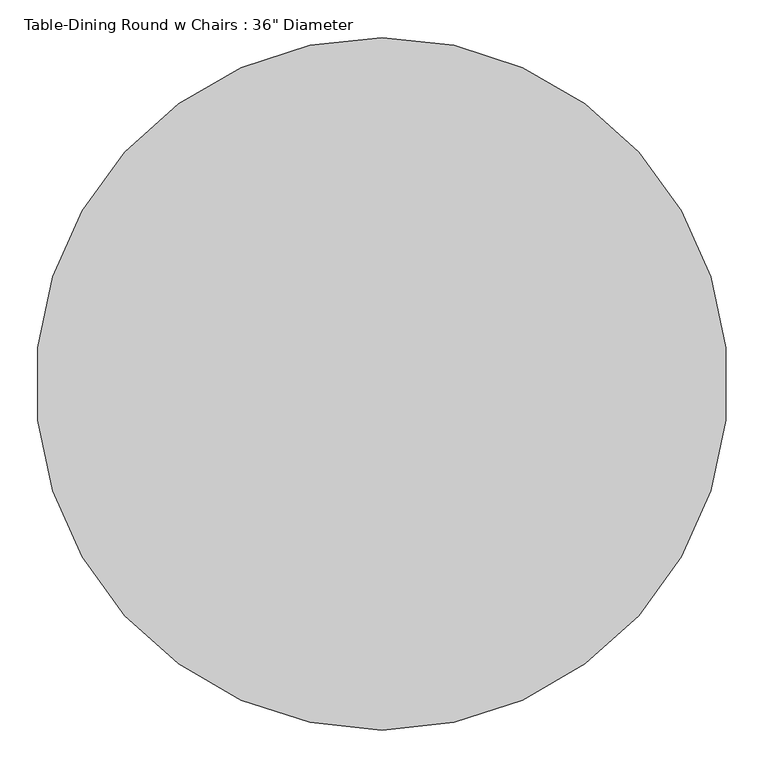
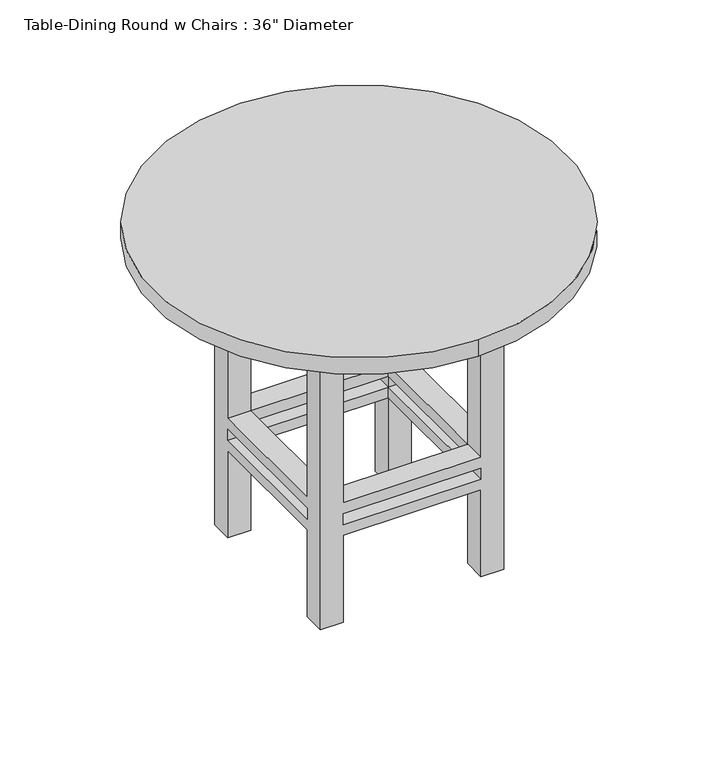
"""IFC4 building model written with IfcOpenShell, lengths in millimetres: furniture geometry."""

from ifc_helpers import new_model, si_unit, point, frame, frame_2d, origin, place, context, project, spatial, polyline, circle_curve, trimmed, segment, composite_curve, outline, extrude, faceted_brep, source, transform, mapped, element, save


def furniture_52f35bf4(model_context):
    return source(origin(), model_context, "Body", "SolidModel", [
        extrude(outline(polyline([(332.2819672, 43.7213115), (332.2819672, -413.4786885), (-124.9180328, -413.4786885), (-124.9180328, 43.7213115), (332.2819672, 43.7213115)]), holes=[polyline([(306.8819672, 18.3213115), (-99.5180328, 18.3213115), (-99.5180328, -388.0786885), (306.8819672, -388.0786885), (306.8819672, 18.3213115)])]), frame((0.0, 0.0, 647.7), z_axis=(0.0, 0.0, 1.0), x_axis=(1.0, 0.0, 0.0)), (0.0, 0.0, 1.0), 76.2),
        faceted_brep([(256.0819672, -32.4786885, 279.4), (256.0819672, -337.2786885, 279.4), (306.8819672, -337.2786885, 279.4), (306.8819672, -32.4786885, 279.4), (-48.7180328, -337.2786885, 279.4), (-48.7180328, -388.0786885, 279.4), (256.0819672, -388.0786885, 279.4), (-48.7180328, -32.4786885, 279.4), (-99.5180328, -32.4786885, 279.4), (-99.5180328, -337.2786885, 279.4), (256.0819672, 18.3213115, 279.4), (-48.7180328, 18.3213115, 279.4), (256.0819672, -32.4786885, 254.0), (-48.7180328, -32.4786885, 254.0), (-48.7180328, 18.3213115, 254.0), (256.0819672, 18.3213115, 254.0), (-48.7180328, -337.2786885, 254.0), (-99.5180328, -337.2786885, 254.0), (-99.5180328, -32.4786885, 254.0), (256.0819672, -337.2786885, 254.0), (256.0819672, -388.0786885, 254.0), (-48.7180328, -388.0786885, 254.0), (306.8819672, -32.4786885, 254.0), (306.8819672, -337.2786885, 254.0), (-99.5180328, 18.3213115, 647.7), (-48.7180328, 18.3213115, 647.7), (256.0819672, 18.3213115, 647.7), (306.8819672, 18.3213115, 647.7), (306.8819672, 18.3213115, 0.0), (256.0819672, 18.3213115, 0.0), (256.0819672, 18.3213115, 203.2), (-48.7180328, 18.3213115, 203.2), (-48.7180328, 18.3213115, 0.0), (-99.5180328, 18.3213115, 0.0), (-48.7180328, 18.3213115, 228.6), (256.0819672, 18.3213115, 228.6), (-99.5180328, -32.4786885, 647.7), (-99.5180328, -32.4786885, 0.0), (-99.5180328, -32.4786885, 203.2), (-99.5180328, -337.2786885, 203.2), (-99.5180328, -337.2786885, 0.0), (-99.5180328, -388.0786885, 0.0), (-99.5180328, -388.0786885, 647.7), (-99.5180328, -337.2786885, 647.7), (-99.5180328, -337.2786885, 228.6), (-99.5180328, -32.4786885, 228.6), (306.8819672, -388.0786885, 647.7), (256.0819672, -388.0786885, 647.7), (-48.7180328, -388.0786885, 647.7), (-48.7180328, -388.0786885, 0.0), (-48.7180328, -388.0786885, 203.2), (256.0819672, -388.0786885, 203.2), (256.0819672, -388.0786885, 0.0), (306.8819672, -388.0786885, 0.0), (256.0819672, -388.0786885, 228.6), (-48.7180328, -388.0786885, 228.6), (306.8819672, -32.4786885, 647.7), (306.8819672, -337.2786885, 647.7), (306.8819672, -337.2786885, 0.0), (306.8819672, -337.2786885, 203.2), (306.8819672, -32.4786885, 203.2), (306.8819672, -32.4786885, 0.0), (306.8819672, -32.4786885, 228.6), (306.8819672, -337.2786885, 228.6), (-48.7180328, -32.4786885, 647.7), (256.0819672, -337.2786885, 647.7), (256.0819672, -32.4786885, 647.7), (-48.7180328, -337.2786885, 647.7), (256.0819672, -32.4786885, 0.0), (-48.7180328, -337.2786885, 0.0), (-48.7180328, -32.4786885, 0.0), (256.0819672, -337.2786885, 0.0), (-48.7180328, -32.4786885, 228.6), (-48.7180328, -32.4786885, 203.2), (256.0819672, -32.4786885, 228.6), (256.0819672, -32.4786885, 203.2), (256.0819672, -337.2786885, 228.6), (256.0819672, -337.2786885, 203.2), (-48.7180328, -337.2786885, 228.6), (-48.7180328, -337.2786885, 203.2)], [[[0, 1, 2, 3]], [[1, 4, 5, 6]], [[4, 7, 8, 9]], [[7, 0, 10, 11]], [[12, 13, 14, 15]], [[13, 16, 17, 18]], [[16, 19, 20, 21]], [[19, 12, 22, 23]], [[24, 25, 11, 10, 26, 27, 28, 29, 30, 31, 32, 33], [14, 34, 35, 15]], [[36, 24, 33, 37, 38, 39, 40, 41, 42, 43, 9, 8], [17, 44, 45, 18]], [[46, 47, 6, 5, 48, 42, 41, 49, 50, 51, 52, 53], [20, 54, 55, 21]], [[28, 27, 56, 3, 2, 57, 46, 53, 58, 59, 60, 61], [22, 62, 63, 23]], [[1, 0, 12, 19]], [[4, 1, 19, 16]], [[7, 4, 16, 13]], [[0, 7, 13, 12]], [[25, 24, 36, 64]], [[47, 46, 57, 65]], [[26, 66, 56, 27]], [[48, 67, 43, 42]], [[29, 28, 61, 68]], [[49, 41, 40, 69]], [[32, 70, 37, 33]], [[52, 71, 58, 53]], [[13, 18, 45, 72]], [[64, 36, 8, 7]], [[37, 70, 73, 38]], [[14, 13, 72, 34]], [[25, 64, 7, 11]], [[70, 32, 31, 73]], [[12, 15, 35, 74]], [[66, 26, 10, 0]], [[29, 68, 75, 30]], [[22, 12, 74, 62]], [[56, 66, 0, 3]], [[68, 61, 60, 75]], [[19, 23, 63, 76]], [[65, 57, 2, 1]], [[58, 71, 77, 59]], [[20, 19, 76, 54]], [[47, 65, 1, 6]], [[71, 52, 51, 77]], [[16, 21, 55, 78]], [[67, 48, 5, 4]], [[49, 69, 79, 50]], [[17, 16, 78, 44]], [[43, 67, 4, 9]], [[69, 40, 39, 79]], [[74, 76, 63, 62]], [[76, 78, 55, 54]], [[78, 72, 45, 44]], [[72, 74, 35, 34]], [[75, 73, 31, 30]], [[73, 79, 39, 38]], [[79, 77, 51, 50]], [[77, 75, 60, 59]], [[76, 74, 75, 77]], [[78, 76, 77, 79]], [[72, 78, 79, 73]], [[74, 72, 73, 75]]]),
        extrude(outline(composite_curve([segment(trimmed(circle_curve(frame_2d((103.6819672, -184.8786885)), 457.2), [point((103.6819672, -642.0786885))], [point((103.6819672, 272.3213115))], False, "CARTESIAN"), True, "CONTINUOUS"), segment(trimmed(circle_curve(frame_2d((103.6819672, -184.8786885)), 457.2), [point((103.6819672, 272.3213115))], [point((103.6819672, -642.0786885))], False, "CARTESIAN"), True, "CONTINUOUS")], self_intersect=False)), frame((0.0, 0.0, 723.9), z_axis=(0.0, 0.0, 1.0), x_axis=(1.0, 0.0, 0.0)), (0.0, 0.0, 1.0), 38.1),
    ])


if __name__ == "__main__":
    model = new_model("IFC4")
    model_context = context("Model", 3, world=origin())
    ifc_project = project(units=[si_unit("LENGTHUNIT", "METRE", prefix="MILLI")], contexts=[model_context])
    site = spatial("IfcSite", under=ifc_project)
    building = spatial("IfcBuilding", under=site)
    placement = place(None, origin())
    furniture_shape = furniture_52f35bf4(model_context)
    element("IfcFurniture", 1, ObjectType="Table-Dining Round w Chairs : 36\" Diameter", at=placement, inside=building, context=model_context, shape_type="MappedRepresentation", body=[
        mapped(furniture_shape, transform((0.0, 0.0, 0.0), x_axis=(1.0, 0.0, 0.0), y_axis=(0.0, 1.0, 0.0), z_axis=(0.0, 0.0, 1.0))),
    ])
    save(model, "model.ifc")

# Revit data of these elements
# Type "Table-Dining Round w Chairs : 36\" Diameter"
#   Assembly Code = "E2020200"
#   Radius = 1.5 ft
#   Diameter = 3 ft
#   Height = 2.5 ft
#   Chairs = 6
#   Base Material = Pine
#   Top Material = Laminate, Linen, Matte
#   Default Elevation = 0
# Element 1 (IfcFurniture, "Table-Dining Round w Chairs : 36\" Diameter")
#   Materials on its faces: "Pine", "Laminate, Linen, Matte"
# Materials
#   "Pine": class "Wood", colour RGB 223 192 134, transparency 0, Description = "Pinus Echinata", Cost = 0
#   "Laminate, Linen, Matte": class "Plastic", colour RGB 249 239 230, transparency 0, Description = "Plastic Laminate - Linen, Matte", Cost = 0
